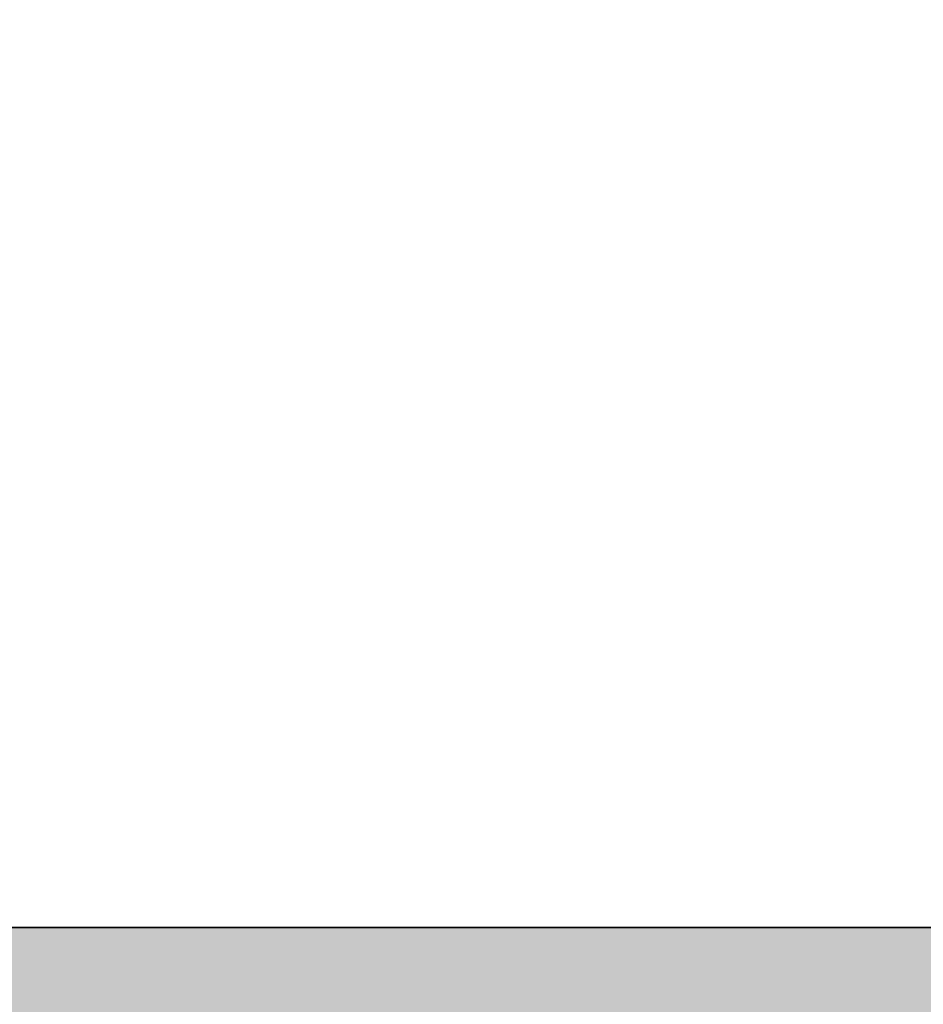
# Model space of a CAD drawing. Units: inches. Extents: x 2696 to 3240, y 1564 to 2310.
# Tile 33 of 76: x 3150.17 to 3160.85, y 1698.79 to 1710.43. Entities that reach past the tile are written whole.
import ezdxf

# ---------------------------------------------------------------- set-up
doc = ezdxf.new("R2010")
doc.units = ezdxf.units.IN
for name, color, linetype, lineweight in [('A-ANNO-DIMS', 3, 'Continuous', 18), ('A-WALL', 7, 'Continuous', 35), ('A-WALL-PATT', 9, 'Continuous', 13)]:
    doc.layers.add(name, color=color, linetype=linetype, lineweight=lineweight)
doc.styles.add('TIMES NEW', font='times.ttf')
doc.dimstyles.new('Siddhuu', dxfattribs={"dimtxt": 6, "dimasz": 2.5, "dimexe": 1.25, "dimexo": 0.625, "dimtad": 1, "dimdec": 1, "dimlunit": 4, "dimtxsty": 'TIMES NEW', "dimcen": 2.5, "dimclrd": 256, "dimclre": 1, "dimclrt": 7, "dimadec": 0, "dimazin": 0, "dimtfac": 1, "dimtdec": 1, "dimtmove": 0, "dimatfit": 3, "dimfxl": 1, "dimtolj": 1, "dimlwd": -1, "dimarcsym": 0})

# ---------------------------------------------------------------- blocks, each defined once
blk = doc.blocks.new('*D52')
at = {"layer": 'A-ANNO-DIMS', "color": 1, "lineweight": -2, "transparency": 16777216}
for p, q in [((3148.611, 1979.576), (3148.611, 1568.951)), ((3190.611, 1979.576), (3190.611, 1568.951))]:
    blk.add_line(p, q, dxfattribs=at)
at = {"layer": 'A-ANNO-DIMS', "transparency": 16777216}
blk.add_line((3151.111, 1570.201), (3188.111, 1570.201), dxfattribs=at)
for points in [[(3151.111, 1570.618), (3151.111, 1569.784), (3148.611, 1570.201)], [(3188.111, 1570.618), (3188.111, 1569.784), (3190.611, 1570.201)]]:
    blk.add_solid(points, dxfattribs=at)
at = {"layer": 'Defpoints', "color": 0, "transparency": 16777216}
for p in [(3148.611, 1980.201), (3190.611, 1980.201), (3190.611, 1570.201)]:
    blk.add_point(p, dxfattribs=at)
at = {"layer": 'A-ANNO-DIMS', "color": 7, "transparency": 16777216, "insert": (3169.611, 1573.878), "char_height": 6, "attachment_point": 5, "style": 'TIMES NEW'}
blk.add_mtext('\\A1;3\'-6"', dxfattribs=at)
blk = doc.blocks.new('*D56')
at = {"layer": 'A-ANNO-DIMS', "color": 1, "lineweight": -2, "transparency": 16777216}
for p, q in [((2966.334, 1884.201), (3235.861, 1884.201)), ((2966.334, 1665.201), (3235.861, 1665.201))]:
    blk.add_line(p, q, dxfattribs=at)
at = {"layer": 'A-ANNO-DIMS', "transparency": 16777216}
blk.add_line((3234.611, 1667.701), (3234.611, 1881.701), dxfattribs=at)
for points in [[(3234.195, 1881.701), (3235.028, 1881.701), (3234.611, 1884.201)], [(3234.195, 1667.701), (3235.028, 1667.701), (3234.611, 1665.201)]]:
    blk.add_solid(points, dxfattribs=at)
at = {"layer": 'Defpoints', "color": 0, "transparency": 16777216}
for p in [(2965.709, 1884.201), (3234.611, 1884.201), (2965.709, 1665.201)]:
    blk.add_point(p, dxfattribs=at)
at = {"layer": 'A-ANNO-DIMS', "color": 7, "transparency": 16777216, "insert": (3230.934, 1774.701), "char_height": 6, "attachment_point": 5, "rotation": 90, "style": 'TIMES NEW'}
blk.add_mtext('\\A1;18\'-3"', dxfattribs=at)

msp = doc.modelspace()

# ---------------------------------------------------------------- hatches: boundary and pattern name
at = {"layer": 'A-WALL-PATT', "transparency": 33554556}
h = msp.add_hatch(color=256, dxfattribs=at)
h.dxf.hatch_style = 1
h.paths.add_polyline_path([(2879.111, 2253.201), (2905.91, 2253.201), (2905.91, 2262.201), (2841.889, 2262.201), (2841.889, 2253.201), (2870.111, 2253.201), (2870.111, 2176.601), (2965.709, 2176.601), (2965.709, 2206.701), (2973.583, 2206.701), (2973.583, 2215.701), (2965.709, 2215.701), (2965.709, 2262.201), (2929.91, 2262.201), (2929.91, 2253.201), (2956.709, 2253.201), (2956.709, 2185.601), (2879.111, 2185.601)])
h.paths.add_polyline_path([(2782.834, 2262.201), (2745.611, 2262.201), (2745.611, 2228.729), (2754.611, 2228.729), (2754.611, 2253.201), (2782.834, 2253.201)])
h.paths.add_polyline_path([(2754.611, 2136.201), (2965.709, 2136.201), (2965.709, 2145.201), (2879.111, 2145.201), (2879.111, 2147.074), (2877.34, 2147.074), (2870.111, 2147.074), (2870.111, 2145.201), (2754.611, 2145.201), (2754.611, 2169.674), (2745.611, 2169.674), (2745.611, 2000.201), (2754.611, 2000.201), (2754.611, 2019.201), (2849.083, 2019.201), (2849.083, 2023.701), (2841.209, 2023.701), (2841.209, 2051.827), (2836.709, 2051.827), (2836.709, 2023.701), (2754.611, 2023.701), (2754.611, 2091.201), (2836.709, 2091.201), (2836.709, 2087.827), (2841.209, 2087.827), (2841.209, 2095.701), (2754.611, 2095.701)])
h.paths.add_polyline_path([(2965.709, 2136.201), (2956.709, 2136.201), (2956.709, 2023.701), (2885.083, 2023.701), (2885.083, 2019.201), (2956.709, 2019.201), (2956.709, 1950.575), (2965.709, 1950.575), (2965.709, 1980.201), (2973.583, 1980.201), (2973.583, 1989.201), (2965.709, 1989.201)])
h.paths.add_polyline_path([(2754.611, 1906.701), (2880.209, 1906.701), (2884.709, 1906.701), (2956.709, 1906.701), (2956.709, 1792.701), (2944.709, 1792.701), (2944.709, 1783.701), (2956.709, 1783.701), (2956.709, 1740.201), (2884.709, 1740.201), (2884.709, 1783.701), (2896.709, 1783.701), (2896.709, 1792.701), (2884.709, 1792.701), (2884.709, 1846.701), (2880.209, 1846.701), (2880.209, 1740.201), (2754.611, 1740.201), (2754.611, 1777.201), (2745.611, 1777.201), (2745.611, 1692.701), (2754.611, 1692.701), (2754.611, 1731.201), (2956.709, 1731.201), (2956.709, 1723.327), (2965.709, 1723.327), (2965.709, 1884.201), (2973.583, 1884.201), (2973.583, 1893.201), (2965.709, 1893.201), (2965.709, 1914.575), (2956.709, 1914.575), (2956.709, 1911.201), (2754.611, 1911.201), (2754.611, 1930.201), (2745.611, 1930.201), (2745.611, 1817.201), (2754.611, 1817.201), (2754.611, 1854.201), (2826.611, 1854.201), (2826.611, 1868.827), (2822.111, 1868.827), (2822.111, 1858.701), (2754.611, 1858.701)])
h.paths.add_polyline_path([(2965.709, 1656.201), (3008.237, 1656.201), (3008.237, 1665.201), (2965.709, 1665.201), (2965.709, 1693.327), (2956.709, 1693.327), (2956.709, 1686.201), (2934.583, 1686.201), (2934.583, 1681.701), (2956.709, 1681.701), (2956.709, 1614.201), (2896.709, 1614.201), (2896.709, 1681.701), (2904.583, 1681.701), (2904.583, 1686.201), (2892.209, 1686.201), (2892.209, 1614.201), (2858.41, 1614.201), (2858.41, 1605.201), (2965.709, 1605.201)])
h.paths.add_polyline_path([(2788.41, 1614.201), (2754.611, 1614.201), (2754.611, 1652.701), (2745.611, 1652.701), (2745.611, 1605.201), (2788.41, 1605.201)])
h.paths.add_polyline_path([(3199.611, 1633.048), (3190.611, 1633.048), (3190.611, 1614.201), (3082.611, 1614.201), (3082.611, 1665.201), (3070.237, 1665.201), (3070.237, 1656.201), (3078.111, 1656.201), (3078.111, 1605.201), (3199.611, 1605.201)])
h.paths.add_polyline_path([(3199.611, 1702.048), (3190.611, 1702.048), (3190.611, 1699.701), (3106.611, 1699.701), (3106.611, 1747.701), (3190.611, 1747.701), (3190.611, 1752.201), (3082.611, 1752.201), (3082.611, 1760.075), (3078.111, 1760.075), (3078.111, 1747.701), (3102.111, 1747.701), (3102.111, 1699.701), (3078.111, 1699.701), (3078.111, 1695.201), (3190.611, 1695.201), (3190.611, 1676.355), (3199.611, 1676.355)])
h.paths.add_polyline_path([(3199.611, 1783.201), (3190.611, 1783.201), (3190.611, 1745.355), (3199.611, 1745.355)])
h.paths.add_polyline_path([(3082.611, 1884.201), (3190.611, 1884.201), (3190.611, 1853.201), (3199.611, 1853.201), (3199.611, 1901.701), (3190.611, 1901.701), (3190.611, 1893.201), (3005.583, 1893.201), (3005.583, 1891.281), (3005.583, 1884.201), (3078.111, 1884.201), (3078.111, 1792.075), (3082.611, 1792.075)])
h.paths.add_polyline_path([(3199.611, 1994.701), (3190.611, 1994.701), (3190.611, 1989.201), (3073.709, 1989.201), (3073.709, 2034.201), (3069.209, 2034.201), (3069.209, 1989.201), (3005.583, 1989.201), (3005.583, 1980.201), (3190.611, 1980.201), (3190.611, 1971.701), (3199.611, 1971.701)])
h.paths.add_polyline_path([(3199.611, 2155.201), (3190.611, 2155.201), (3190.611, 2064.701), (3199.611, 2064.701)])
h.paths.add_polyline_path([(3190.611, 2074.701), (3106.611, 2074.701), (3106.611, 2122.701), (3190.611, 2122.701), (3190.611, 2127.201), (3082.709, 2127.201), (3082.709, 2135.075), (3073.709, 2135.075), (3073.709, 2122.701), (3102.111, 2122.701), (3102.111, 2074.701), (3069.209, 2074.701), (3069.209, 2070.201), (3190.611, 2070.201)])
h.paths.add_polyline_path([(3082.709, 2253.201), (3190.611, 2253.201), (3190.611, 2225.201), (3199.611, 2225.201), (3199.611, 2262.201), (3073.709, 2262.201), (3073.709, 2215.701), (3035.583, 2215.701), (3035.583, 2206.701), (3073.709, 2206.701), (3073.709, 2171.075), (3082.709, 2171.075)])

# ---------------------------------------------------------------- linework, layer by layer
at = {"layer": 'A-WALL'}
msp.add_line((3106.611, 1699.701), (3190.611, 1699.701), dxfattribs=at)

# ---------------------------------------------------------------- dimensions: what is measured, and where the dimension line sits
at = {"layer": 'A-ANNO-DIMS'}
dim = msp.add_linear_dim(base=(3190.611, 1570.201), p1=(3148.611, 1980.201), p2=(3190.611, 1980.201), dimstyle='Siddhuu', override={"dimdec": 1, "dimlfac": 1, "dimrnd": 0, "dimzin": 1, "dimdsep": 46, "dimlunit": 4, "dimfrac": 2}, dxfattribs=at)
dim.commit()
dim.dimension.update_dxf_attribs({"geometry": '*D52', "text_midpoint": (3169.611, 1573.878)})
dim = msp.add_linear_dim(base=(3234.611, 1884.201), p1=(2965.709, 1665.201), p2=(2965.709, 1884.201), angle=90, dimstyle='Siddhuu', override={"dimdec": 1, "dimlfac": 1, "dimrnd": 0, "dimzin": 1, "dimdsep": 46, "dimlunit": 4, "dimfrac": 2}, dxfattribs=at)
dim.commit()
dim.dimension.update_dxf_attribs({"geometry": '*D56', "text_midpoint": (3230.934, 1774.701)})

doc.saveas('drawing.dxf')
